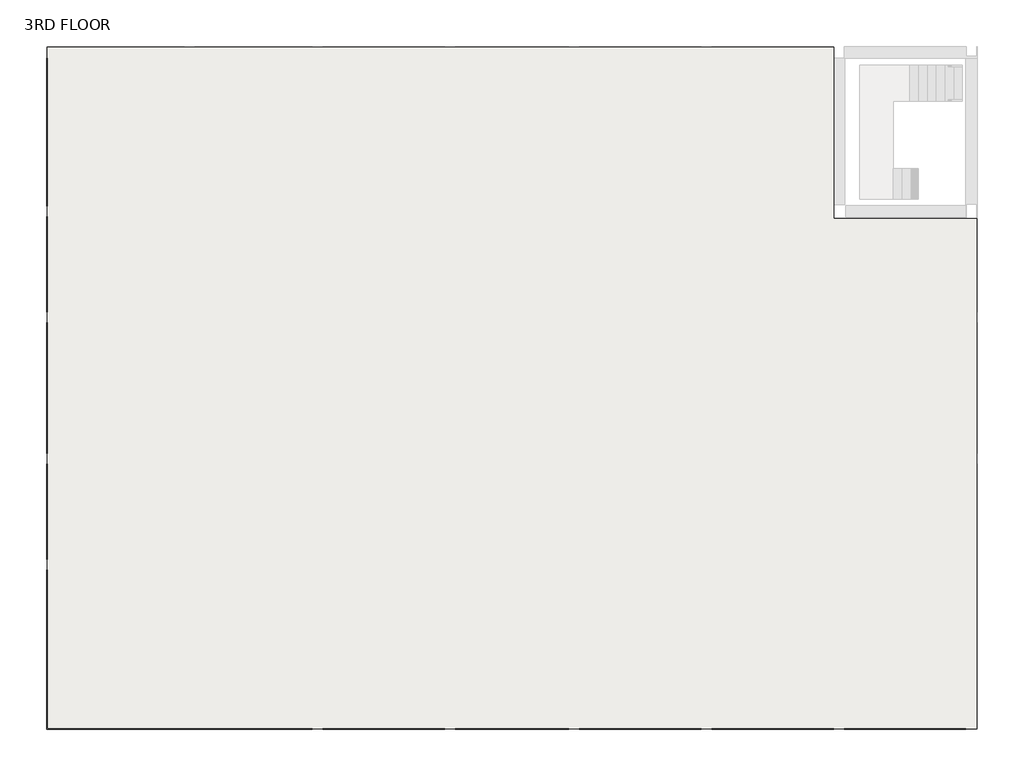
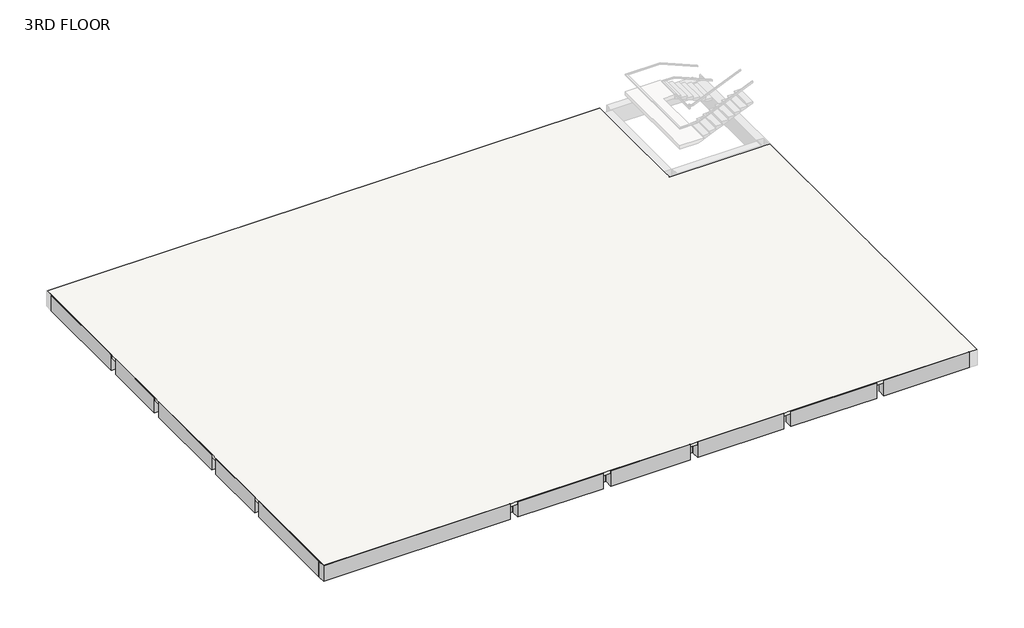
# One storey, part 1 of 2: 9 beams, 1 slab.
"""IFC4 building model written with IfcOpenShell, lengths in millimetres."""

from ifc_helpers import new_model, si_unit, frame, origin, place, context, project, spatial, polyline, outline, extrude, faceted_brep, element, save

model = new_model("IFC4")

# Units and contexts
model_context = context("Model", 3, world=origin())
ifc_project = project(units=[si_unit("LENGTHUNIT", "METRE", prefix="MILLI")], contexts=[model_context])

# Site, building, storey
site = spatial("IfcSite", under=ifc_project)
building = spatial("IfcBuilding", under=site)
storey = spatial("IfcBuildingStorey", under=building, Name="3RD FLOOR", Elevation=10668.0)

# Beams
placement = place(None, origin())
element("IfcBeam", 1, ObjectType="M_Concrete-Rectangular Beam : 400 x 800mm", at=placement, inside=storey, context=model_context, shape_type="Brep", body=[
    faceted_brep([(-25701.5491019, -6047.8309165, 10668.0), (-25701.5491019, -6447.8309165, 10668.0), (-16535.3491019, -6447.8309165, 10668.0), (-16535.3491019, -6425.6309165, 10668.0), (-25679.3491019, -6425.6309165, 10668.0), (-25679.3491019, -6047.8309165, 10668.0), (-25701.5491019, -6047.8309165, 9868.0), (-25679.3491019, -6047.8309165, 10515.6), (-25301.5491019, -6047.8309165, 10515.6), (-20977.1491019, -6047.8309165, 10515.6), (-20577.1491019, -6047.8309165, 10515.6), (-16557.5491019, -6047.8309165, 10515.6), (-16535.3491019, -6047.8309165, 10515.6), (-16535.3491019, -6047.8309165, 9868.0), (-16557.5491019, -6047.8309165, 9868.0), (-20577.1491019, -6047.8309165, 9868.0), (-20977.1491019, -6047.8309165, 9868.0), (-25301.5491019, -6047.8309165, 9868.0), (-25701.5491019, -6447.8309165, 9868.0), (-16535.3491019, -6447.8309165, 9868.0), (-25323.7491019, -6425.6309165, 9868.0), (-25323.7491019, -6070.0309165, 9868.0), (-25679.3491019, -6070.0309165, 9868.0), (-25679.3491019, -6425.6309165, 9868.0), (-20599.3491019, -6425.6309165, 9868.0), (-20599.3491019, -6070.0309165, 9868.0), (-20954.9491019, -6070.0309165, 9868.0), (-20954.9491019, -6425.6309165, 9868.0), (-25323.7491019, -6425.6309165, 10515.6), (-25323.7491019, -6070.0309165, 10515.6), (-16535.3491019, -6425.6309165, 10515.6), (-20599.3491019, -6425.6309165, 10515.6), (-20954.9491019, -6425.6309165, 10515.6), (-25679.3491019, -6425.6309165, 10515.6), (-25679.3491019, -6070.0309165, 10515.6), (-20599.3491019, -6070.0309165, 10515.6), (-20954.9491019, -6070.0309165, 10515.6)], [[[0, 1, 2, 3, 4, 5]], [[6, 0, 5, 7, 8, 9, 10, 11, 12, 13, 14, 15, 16, 17]], [[18, 6, 17, 16, 15, 14, 13, 19], [20, 21, 22, 23], [24, 25, 26, 27]], [[1, 18, 19, 2]], [[1, 0, 6, 18]], [[21, 20, 28, 29]], [[30, 31, 24, 27, 32, 28, 20, 23, 33, 4, 3]], [[4, 33, 23, 22, 34, 7, 5]], [[22, 21, 29, 34]], [[25, 24, 31, 35]], [[27, 26, 36, 32]], [[26, 25, 35, 36]], [[19, 13, 12, 30, 3, 2]], [[28, 32, 36, 35, 31, 30, 12, 11, 10, 9, 8, 7, 34, 29]]]),
    faceted_brep([(5997.6508981, -6447.8309165, 9868.0), (5997.6508981, -6047.8309165, 9868.0), (5997.6508981, -6047.8309165, 10515.6), (5997.6508981, -6425.6309165, 10515.6), (5997.6508981, -6425.6309165, 10668.0), (5997.6508981, -6447.8309165, 10668.0), (1803.4508981, -6047.8309165, 9868.0), (1803.4508981, -6447.8309165, 9868.0), (1803.4508981, -6447.8309165, 10668.0), (1803.4508981, -6425.6309165, 10668.0), (1803.4508981, -6425.6309165, 10515.6), (1803.4508981, -6047.8309165, 10515.6), (1825.6508981, -6047.8309165, 9868.0), (1825.6508981, -6047.8309165, 10515.6)], [[[0, 1, 2, 3, 4, 5]], [[6, 7, 8, 9, 10, 11]], [[8, 5, 4, 9]], [[1, 12, 6, 11, 13, 2]], [[1, 0, 7, 6, 12]], [[0, 5, 8, 7]], [[10, 3, 2, 13, 11]], [[3, 10, 9, 4]]]),
    faceted_brep([(-16179.7491019, -6047.8309165, 9868.0), (-16179.7491019, -6447.8309165, 9868.0), (-16179.7491019, -6447.8309165, 10668.0), (-16179.7491019, -6425.6309165, 10668.0), (-16179.7491019, -6425.6309165, 10515.6), (-16179.7491019, -6047.8309165, 10515.6), (-11963.3491019, -6447.8309165, 10668.0), (-11963.3491019, -6425.6309165, 10668.0), (-11963.3491019, -6047.8309165, 9868.0), (-11985.5491019, -6047.8309165, 9868.0), (-16157.5491019, -6047.8309165, 9868.0), (-16157.5491019, -6047.8309165, 10515.6), (-11985.5491019, -6047.8309165, 10515.6), (-11963.3491019, -6047.8309165, 10515.6), (-11963.3491019, -6447.8309165, 9868.0), (-11963.3491019, -6425.6309165, 10515.6)], [[[0, 1, 2, 3, 4, 5]], [[2, 6, 7, 3]], [[8, 9, 10, 0, 5, 11, 12, 13]], [[1, 0, 10, 9, 8, 14]], [[2, 1, 14, 6]], [[14, 8, 13, 15, 7, 6]], [[15, 4, 3, 7]], [[4, 15, 13, 12, 11, 5]]]),
    faceted_brep([(-11607.7491019, -6047.8309165, 9868.0), (-11607.7491019, -6447.8309165, 9868.0), (-11607.7491019, -6447.8309165, 10668.0), (-11607.7491019, -6425.6309165, 10668.0), (-11607.7491019, -6425.6309165, 10515.6), (-11607.7491019, -6047.8309165, 10515.6), (-7696.1491019, -6447.8309165, 10668.0), (-7696.1491019, -6425.6309165, 10668.0), (-7696.1491019, -6047.8309165, 9868.0), (-7718.3491019, -6047.8309165, 9868.0), (-11585.5491019, -6047.8309165, 9868.0), (-11585.5491019, -6047.8309165, 10515.6), (-7718.3491019, -6047.8309165, 10515.6), (-7696.1491019, -6047.8309165, 10515.6), (-7696.1491019, -6447.8309165, 9868.0), (-7696.1491019, -6425.6309165, 10515.6)], [[[0, 1, 2, 3, 4, 5]], [[2, 6, 7, 3]], [[8, 9, 10, 0, 5, 11, 12, 13]], [[1, 0, 10, 9, 8, 14]], [[2, 1, 14, 6]], [[14, 8, 13, 15, 7, 6]], [[15, 4, 3, 7]], [[4, 15, 13, 12, 11, 5]]]),
    faceted_brep([(-7340.5491019, -6047.8309165, 9868.0), (-7340.5491019, -6447.8309165, 9868.0), (-7340.5491019, -6447.8309165, 10668.0), (-7340.5491019, -6425.6309165, 10668.0), (-7340.5491019, -6425.6309165, 10515.6), (-7340.5491019, -6047.8309165, 10515.6), (-3124.1491019, -6447.8309165, 10668.0), (-3124.1491019, -6425.6309165, 10668.0), (-3124.1491019, -6047.8309165, 9868.0), (-3146.3491019, -6047.8309165, 9868.0), (-7318.3491019, -6047.8309165, 9868.0), (-7318.3491019, -6047.8309165, 10515.6), (-3146.3491019, -6047.8309165, 10515.6), (-3124.1491019, -6047.8309165, 10515.6), (-3124.1491019, -6447.8309165, 9868.0), (-3124.1491019, -6425.6309165, 10515.6)], [[[0, 1, 2, 3, 4, 5]], [[2, 6, 7, 3]], [[8, 9, 10, 0, 5, 11, 12, 13]], [[1, 0, 10, 9, 8, 14]], [[2, 1, 14, 6]], [[14, 8, 13, 15, 7, 6]], [[15, 4, 3, 7]], [[4, 15, 13, 12, 11, 5]]]),
    faceted_brep([(-2768.5491019, -6047.8309165, 9868.0), (-2768.5491019, -6447.8309165, 9868.0), (-2768.5491019, -6447.8309165, 10668.0), (-2768.5491019, -6425.6309165, 10668.0), (-2768.5491019, -6425.6309165, 10515.6), (-2768.5491019, -6047.8309165, 10515.6), (1447.8508981, -6447.8309165, 10668.0), (1447.8508981, -6425.6309165, 10668.0), (1447.8508981, -6047.8309165, 9868.0), (1425.6508981, -6047.8309165, 9868.0), (-2746.3491019, -6047.8309165, 9868.0), (-2746.3491019, -6047.8309165, 10515.6), (1425.6508981, -6047.8309165, 10515.6), (1447.8508981, -6047.8309165, 10515.6), (1447.8508981, -6447.8309165, 9868.0), (1447.8508981, -6425.6309165, 10515.6)], [[[0, 1, 2, 3, 4, 5]], [[2, 6, 7, 3]], [[8, 9, 10, 0, 5, 11, 12, 13]], [[1, 0, 10, 9, 8, 14]], [[2, 1, 14, 6]], [[14, 8, 13, 15, 7, 6]], [[15, 4, 3, 7]], [[4, 15, 13, 12, 11, 5]]]),
])
element("IfcBeam", 2, ObjectType="M_Concrete-Rectangular Beam : 400 x 800mm", at=placement, inside=storey, context=model_context, shape_type="Brep", body=[
    faceted_brep([(-25701.5491019, -939.2309165, 10668.0), (-25701.5491019, -6047.8309165, 10668.0), (-25679.3491019, -6047.8309165, 10668.0), (-25679.3491019, -939.2309165, 10668.0), (-25301.5491019, -6047.8309165, 9868.0), (-25301.5491019, -961.4309165, 9868.0), (-25301.5491019, -939.2309165, 9868.0), (-25301.5491019, -939.2309165, 10515.6), (-25301.5491019, -961.4309165, 10515.6), (-25301.5491019, -6047.8309165, 10515.6), (-25701.5491019, -6047.8309165, 9868.0), (-25701.5491019, -939.2309165, 9868.0), (-25679.3491019, -6047.8309165, 10515.6), (-25679.3491019, -939.2309165, 10515.6)], [[[0, 1, 2, 3]], [[4, 5, 6, 7, 8, 9]], [[4, 10, 11, 6, 5]], [[10, 1, 0, 11]], [[10, 4, 9, 12, 2, 1]], [[6, 11, 0, 3, 13, 7]], [[12, 13, 3, 2]], [[13, 12, 9, 8, 7]]]),
    faceted_brep([(-25301.5491019, 16716.9690835, 9868.0), (-25701.5491019, 16716.9690835, 9868.0), (-25701.5491019, 16716.9690835, 10668.0), (-25679.3491019, 16716.9690835, 10668.0), (-25679.3491019, 16716.9690835, 10515.6), (-25301.5491019, 16716.9690835, 10515.6), (-25701.5491019, 11608.3690835, 10668.0), (-25679.3491019, 11608.3690835, 10668.0), (-25301.5491019, 11608.3690835, 9868.0), (-25301.5491019, 11630.5690835, 9868.0), (-25301.5491019, 11630.5690835, 10515.6), (-25301.5491019, 11608.3690835, 10515.6), (-25701.5491019, 11608.3690835, 9868.0), (-25679.3491019, 11608.3690835, 10515.6)], [[[0, 1, 2, 3, 4, 5]], [[2, 6, 7, 3]], [[8, 9, 0, 5, 10, 11]], [[1, 0, 9, 8, 12]], [[2, 1, 12, 6]], [[12, 8, 11, 13, 7, 6]], [[4, 13, 11, 10, 5]], [[13, 4, 3, 7]]]),
    faceted_brep([(-25701.5491019, 7950.7690835, 9868.0), (-25301.5491019, 7950.7690835, 9868.0), (-25301.5491019, 7950.7690835, 10515.6), (-25679.3491019, 7950.7690835, 10515.6), (-25679.3491019, 7950.7690835, 10668.0), (-25701.5491019, 7950.7690835, 10668.0), (-25301.5491019, 11252.7690835, 9868.0), (-25701.5491019, 11252.7690835, 9868.0), (-25701.5491019, 11252.7690835, 10668.0), (-25679.3491019, 11252.7690835, 10668.0), (-25679.3491019, 11252.7690835, 10515.6), (-25301.5491019, 11252.7690835, 10515.6), (-25301.5491019, 7972.9690835, 10515.6), (-25301.5491019, 11230.5690835, 10515.6), (-25301.5491019, 7972.9690835, 9868.0), (-25301.5491019, 11230.5690835, 9868.0)], [[[0, 1, 2, 3, 4, 5]], [[6, 7, 8, 9, 10, 11]], [[10, 3, 2, 12, 13, 11]], [[3, 10, 9, 4]], [[8, 5, 4, 9]], [[1, 14, 15, 6, 11, 13, 12, 2]], [[1, 0, 7, 6, 15, 14]], [[0, 5, 8, 7]]]),
    faceted_brep([(-25301.5491019, 7595.1690835, 9868.0), (-25701.5491019, 7595.1690835, 9868.0), (-25701.5491019, 7595.1690835, 10668.0), (-25679.3491019, 7595.1690835, 10668.0), (-25679.3491019, 7595.1690835, 10515.6), (-25301.5491019, 7595.1690835, 10515.6), (-25701.5491019, 3073.9690835, 9868.0), (-25301.5491019, 3073.9690835, 9868.0), (-25301.5491019, 3073.9690835, 10515.6), (-25679.3491019, 3073.9690835, 10515.6), (-25679.3491019, 3073.9690835, 10668.0), (-25701.5491019, 3073.9690835, 10668.0), (-25301.5491019, 3096.1690835, 10515.6), (-25301.5491019, 7572.9690835, 10515.6), (-25301.5491019, 3096.1690835, 9868.0), (-25301.5491019, 7572.9690835, 9868.0)], [[[0, 1, 2, 3, 4, 5]], [[6, 7, 8, 9, 10, 11]], [[4, 9, 8, 12, 13, 5]], [[9, 4, 3, 10]], [[2, 11, 10, 3]], [[7, 14, 15, 0, 5, 13, 12, 8]], [[1, 0, 15, 14, 7, 6]], [[2, 1, 6, 11]]]),
    faceted_brep([(-25301.5491019, 2718.3690835, 9868.0), (-25701.5491019, 2718.3690835, 9868.0), (-25701.5491019, 2718.3690835, 10668.0), (-25679.3491019, 2718.3690835, 10668.0), (-25679.3491019, 2718.3690835, 10515.6), (-25301.5491019, 2718.3690835, 10515.6), (-25701.5491019, -583.6309165, 9868.0), (-25301.5491019, -583.6309165, 9868.0), (-25301.5491019, -583.6309165, 10515.6), (-25679.3491019, -583.6309165, 10515.6), (-25679.3491019, -583.6309165, 10668.0), (-25701.5491019, -583.6309165, 10668.0), (-25301.5491019, -561.4309165, 10515.6), (-25301.5491019, 2696.1690835, 10515.6), (-25301.5491019, -561.4309165, 9868.0), (-25301.5491019, 2696.1690835, 9868.0)], [[[0, 1, 2, 3, 4, 5]], [[6, 7, 8, 9, 10, 11]], [[4, 9, 8, 12, 13, 5]], [[9, 4, 3, 10]], [[2, 11, 10, 3]], [[7, 14, 15, 0, 5, 13, 12, 8]], [[0, 15, 14, 7, 6, 1]], [[11, 2, 1, 6]]]),
])
element("IfcBeam", 3, ObjectType="M_Concrete-Rectangular Beam : 400 x 800mm", at=placement, inside=storey, context=model_context, shape_type="SweptSolid", body=[
    extrude(outline(polyline([(-20577.1491019, -6047.8309165), (-20977.1491019, -6047.8309165), (-20977.1491019, -990.0309165), (-20577.1491019, -990.0309165), (-20577.1491019, -6047.8309165)])), frame((0.0, 0.0, 9868.0), z_axis=(0.0, 0.0, 1.0), x_axis=(1.0, 0.0, 0.0)), (0.0, 0.0, 1.0), 647.6),
    extrude(outline(polyline([(-20599.3491019, 16716.9690835), (-20577.1491019, 16716.9690835), (-20577.1491019, 11659.1690835), (-20977.1491019, 11659.1690835), (-20977.1491019, 16716.9690835), (-20954.9491019, 16716.9690835), (-20954.9491019, 16662.9690835), (-20599.3491019, 16662.9690835), (-20599.3491019, 16716.9690835)])), frame((0.0, 0.0, 9868.0), z_axis=(0.0, 0.0, 1.0), x_axis=(1.0, 0.0, 0.0)), (0.0, 0.0, 1.0), 647.6),
    extrude(outline(polyline([(-20977.1491019, 11201.9690835), (-20577.1491019, 11201.9690835), (-20577.1491019, 8001.5690835), (-20977.1491019, 8001.5690835), (-20977.1491019, 11201.9690835)])), frame((0.0, 0.0, 9868.0), z_axis=(0.0, 0.0, 1.0), x_axis=(1.0, 0.0, 0.0)), (0.0, 0.0, 1.0), 647.6),
    extrude(outline(polyline([(-20977.1491019, 7544.3690835), (-20577.1491019, 7544.3690835), (-20577.1491019, 3124.7690835), (-20977.1491019, 3124.7690835), (-20977.1491019, 7544.3690835)])), frame((0.0, 0.0, 9868.0), z_axis=(0.0, 0.0, 1.0), x_axis=(1.0, 0.0, 0.0)), (0.0, 0.0, 1.0), 647.6),
    extrude(outline(polyline([(-20977.1491019, 2667.5690835), (-20577.1491019, 2667.5690835), (-20577.1491019, -532.8309165), (-20977.1491019, -532.8309165), (-20977.1491019, 2667.5690835)])), frame((0.0, 0.0, 9868.0), z_axis=(0.0, 0.0, 1.0), x_axis=(1.0, 0.0, 0.0)), (0.0, 0.0, 1.0), 647.6),
])
element("IfcBeam", 4, ObjectType="M_Concrete-Rectangular Beam : 400 x 800mm", at=placement, inside=storey, context=model_context, shape_type="SweptSolid", body=[
    extrude(outline(polyline([(-16157.5491019, -6047.8309165), (-16179.7491019, -6047.8309165), (-16179.7491019, -6019.2309165), (-16535.3491019, -6019.2309165), (-16535.3491019, -6047.8309165), (-16557.5491019, -6047.8309165), (-16557.5491019, -990.0309165), (-16157.5491019, -990.0309165), (-16157.5491019, -6047.8309165)])), frame((0.0, 0.0, 9868.0), z_axis=(0.0, 0.0, 1.0), x_axis=(1.0, 0.0, 0.0)), (0.0, 0.0, 1.0), 647.6),
    extrude(outline(polyline([(-16179.7491019, 16716.9690835), (-16157.5491019, 16716.9690835), (-16157.5491019, 11659.1690835), (-16557.5491019, 11659.1690835), (-16557.5491019, 16716.9690835), (-16535.3491019, 16716.9690835), (-16535.3491019, 16688.3690835), (-16179.7491019, 16688.3690835), (-16179.7491019, 16716.9690835)])), frame((0.0, 0.0, 9868.0), z_axis=(0.0, 0.0, 1.0), x_axis=(1.0, 0.0, 0.0)), (0.0, 0.0, 1.0), 647.6),
    extrude(outline(polyline([(-16557.5491019, 11201.9690835), (-16157.5491019, 11201.9690835), (-16157.5491019, 8001.5690835), (-16557.5491019, 8001.5690835), (-16557.5491019, 11201.9690835)])), frame((0.0, 0.0, 9868.0), z_axis=(0.0, 0.0, 1.0), x_axis=(1.0, 0.0, 0.0)), (0.0, 0.0, 1.0), 647.6),
    extrude(outline(polyline([(-16557.5491019, 7544.3690835), (-16157.5491019, 7544.3690835), (-16157.5491019, 3124.7690835), (-16557.5491019, 3124.7690835), (-16557.5491019, 7544.3690835)])), frame((0.0, 0.0, 9868.0), z_axis=(0.0, 0.0, 1.0), x_axis=(1.0, 0.0, 0.0)), (0.0, 0.0, 1.0), 647.6),
    extrude(outline(polyline([(-16557.5491019, 2667.5690835), (-16157.5491019, 2667.5690835), (-16157.5491019, -532.8309165), (-16557.5491019, -532.8309165), (-16557.5491019, 2667.5690835)])), frame((0.0, 0.0, 9868.0), z_axis=(0.0, 0.0, 1.0), x_axis=(1.0, 0.0, 0.0)), (0.0, 0.0, 1.0), 647.6),
])
element("IfcBeam", 5, ObjectType="M_Concrete-Rectangular Beam : 400 x 800mm", at=placement, inside=storey, context=model_context, shape_type="SweptSolid", body=[
    extrude(outline(polyline([(-11585.5491019, -6047.8309165), (-11607.7491019, -6047.8309165), (-11607.7491019, -6019.2309165), (-11963.3491019, -6019.2309165), (-11963.3491019, -6047.8309165), (-11985.5491019, -6047.8309165), (-11985.5491019, -990.0309165), (-11585.5491019, -990.0309165), (-11585.5491019, -6047.8309165)])), frame((0.0, 0.0, 9868.0), z_axis=(0.0, 0.0, 1.0), x_axis=(1.0, 0.0, 0.0)), (0.0, 0.0, 1.0), 647.6),
    extrude(outline(polyline([(-11607.7491019, 16716.9690835), (-11585.5491019, 16716.9690835), (-11585.5491019, 11659.1690835), (-11985.5491019, 11659.1690835), (-11985.5491019, 16716.9690835), (-11963.3491019, 16716.9690835), (-11963.3491019, 16688.3690835), (-11607.7491019, 16688.3690835), (-11607.7491019, 16716.9690835)])), frame((0.0, 0.0, 9868.0), z_axis=(0.0, 0.0, 1.0), x_axis=(1.0, 0.0, 0.0)), (0.0, 0.0, 1.0), 647.6),
    extrude(outline(polyline([(-11985.5491019, 11201.9690835), (-11585.5491019, 11201.9690835), (-11585.5491019, 8001.5690835), (-11985.5491019, 8001.5690835), (-11985.5491019, 11201.9690835)])), frame((0.0, 0.0, 9868.0), z_axis=(0.0, 0.0, 1.0), x_axis=(1.0, 0.0, 0.0)), (0.0, 0.0, 1.0), 647.6),
    extrude(outline(polyline([(-11985.5491019, 7544.3690835), (-11585.5491019, 7544.3690835), (-11585.5491019, 3124.7690835), (-11985.5491019, 3124.7690835), (-11985.5491019, 7544.3690835)])), frame((0.0, 0.0, 9868.0), z_axis=(0.0, 0.0, 1.0), x_axis=(1.0, 0.0, 0.0)), (0.0, 0.0, 1.0), 647.6),
    extrude(outline(polyline([(-11585.5491019, -532.8309165), (-11985.5491019, -532.8309165), (-11985.5491019, 2667.5690835), (-11585.5491019, 2667.5690835), (-11585.5491019, -532.8309165)])), frame((0.0, 0.0, 9868.0), z_axis=(0.0, 0.0, 1.0), x_axis=(1.0, 0.0, 0.0)), (0.0, 0.0, 1.0), 647.6),
])
element("IfcBeam", 6, ObjectType="M_Concrete-Rectangular Beam : 400 x 800mm", at=placement, inside=storey, context=model_context, shape_type="SweptSolid", body=[
    extrude(outline(polyline([(-7318.3491019, -6047.8309165), (-7340.5491019, -6047.8309165), (-7340.5491019, -6019.2309165), (-7696.1491019, -6019.2309165), (-7696.1491019, -6047.8309165), (-7718.3491019, -6047.8309165), (-7718.3491019, -990.0309165), (-7318.3491019, -990.0309165), (-7318.3491019, -6047.8309165)])), frame((0.0, 0.0, 9868.0), z_axis=(0.0, 0.0, 1.0), x_axis=(1.0, 0.0, 0.0)), (0.0, 0.0, 1.0), 647.6),
    extrude(outline(polyline([(-7340.5491019, 16716.9690835), (-7318.3491019, 16716.9690835), (-7318.3491019, 11659.1690835), (-7718.3491019, 11659.1690835), (-7718.3491019, 16716.9690835), (-7696.1491019, 16716.9690835), (-7696.1491019, 16688.3690835), (-7340.5491019, 16688.3690835), (-7340.5491019, 16716.9690835)])), frame((0.0, 0.0, 9868.0), z_axis=(0.0, 0.0, 1.0), x_axis=(1.0, 0.0, 0.0)), (0.0, 0.0, 1.0), 647.6),
    extrude(outline(polyline([(-7718.3491019, 7544.3690835), (-7318.3491019, 7544.3690835), (-7318.3491019, 3124.7690835), (-7718.3491019, 3124.7690835), (-7718.3491019, 7544.3690835)])), frame((0.0, 0.0, 9868.0), z_axis=(0.0, 0.0, 1.0), x_axis=(1.0, 0.0, 0.0)), (0.0, 0.0, 1.0), 647.6),
    extrude(outline(polyline([(-7318.3491019, 8001.5690835), (-7718.3491019, 8001.5690835), (-7718.3491019, 11201.9690835), (-7318.3491019, 11201.9690835), (-7318.3491019, 8001.5690835)])), frame((0.0, 0.0, 9868.0), z_axis=(0.0, 0.0, 1.0), x_axis=(1.0, 0.0, 0.0)), (0.0, 0.0, 1.0), 647.6),
    extrude(outline(polyline([(-7318.3491019, -532.8309165), (-7718.3491019, -532.8309165), (-7718.3491019, 2667.5690835), (-7318.3491019, 2667.5690835), (-7318.3491019, -532.8309165)])), frame((0.0, 0.0, 9868.0), z_axis=(0.0, 0.0, 1.0), x_axis=(1.0, 0.0, 0.0)), (0.0, 0.0, 1.0), 647.6),
])
element("IfcBeam", 7, ObjectType="M_Concrete-Rectangular Beam : 400 x 800mm", at=placement, inside=storey, context=model_context, shape_type="SweptSolid", body=[
    extrude(outline(polyline([(-25301.5491019, 3073.9690835), (-25301.5491019, 3096.1690835), (-21005.7491019, 3096.1690835), (-21005.7491019, 2696.1690835), (-25301.5491019, 2696.1690835), (-25301.5491019, 2718.3690835), (-25272.9491019, 2718.3690835), (-25272.9491019, 3073.9690835), (-25301.5491019, 3073.9690835)])), frame((0.0, 0.0, 9868.0), z_axis=(0.0, 0.0, 1.0), x_axis=(1.0, 0.0, 0.0)), (0.0, 0.0, 1.0), 647.6),
    extrude(outline(polyline([(5997.6508981, 3096.1690835), (5997.6508981, 3073.9690835), (5969.0508981, 3073.9690835), (5969.0508981, 2718.3690835), (5997.6508981, 2718.3690835), (5997.6508981, 2696.1690835), (1854.2508981, 2696.1690835), (1854.2508981, 3096.1690835), (5997.6508981, 3096.1690835)])), frame((0.0, 0.0, 9868.0), z_axis=(0.0, 0.0, 1.0), x_axis=(1.0, 0.0, 0.0)), (0.0, 0.0, 1.0), 647.6),
    extrude(outline(polyline([(-20548.5491019, 2696.1690835), (-20548.5491019, 3096.1690835), (-16586.1491019, 3096.1690835), (-16586.1491019, 2696.1690835), (-20548.5491019, 2696.1690835)])), frame((0.0, 0.0, 9868.0), z_axis=(0.0, 0.0, 1.0), x_axis=(1.0, 0.0, 0.0)), (0.0, 0.0, 1.0), 647.6),
    extrude(outline(polyline([(-16128.9491019, 2696.1690835), (-16128.9491019, 3096.1690835), (-12014.1491019, 3096.1690835), (-12014.1491019, 2696.1690835), (-16128.9491019, 2696.1690835)])), frame((0.0, 0.0, 9868.0), z_axis=(0.0, 0.0, 1.0), x_axis=(1.0, 0.0, 0.0)), (0.0, 0.0, 1.0), 647.6),
    extrude(outline(polyline([(1397.0508981, 3096.1690835), (1397.0508981, 2696.1690835), (-2717.7491019, 2696.1690835), (-2717.7491019, 3096.1690835), (1397.0508981, 3096.1690835)])), frame((0.0, 0.0, 9868.0), z_axis=(0.0, 0.0, 1.0), x_axis=(1.0, 0.0, 0.0)), (0.0, 0.0, 1.0), 647.6),
    extrude(outline(polyline([(-3174.9491019, 3096.1690835), (-3174.9491019, 2696.1690835), (-7289.7491019, 2696.1690835), (-7289.7491019, 3096.1690835), (-3174.9491019, 3096.1690835)])), frame((0.0, 0.0, 9868.0), z_axis=(0.0, 0.0, 1.0), x_axis=(1.0, 0.0, 0.0)), (0.0, 0.0, 1.0), 647.6),
    extrude(outline(polyline([(-7746.9491019, 3096.1690835), (-7746.9491019, 2696.1690835), (-11556.9491019, 2696.1690835), (-11556.9491019, 3096.1690835), (-7746.9491019, 3096.1690835)])), frame((0.0, 0.0, 9868.0), z_axis=(0.0, 0.0, 1.0), x_axis=(1.0, 0.0, 0.0)), (0.0, 0.0, 1.0), 647.6),
])
element("IfcBeam", 8, ObjectType="M_Concrete-Rectangular Beam : 400 x 800mm", at=placement, inside=storey, context=model_context, shape_type="SweptSolid", body=[
    extrude(outline(polyline([(-25301.5491019, -583.6309165), (-25301.5491019, -561.4309165), (-21005.7491019, -561.4309165), (-21005.7491019, -961.4309165), (-25301.5491019, -961.4309165), (-25301.5491019, -939.2309165), (-25247.5491019, -939.2309165), (-25247.5491019, -583.6309165), (-25301.5491019, -583.6309165)])), frame((0.0, 0.0, 9868.0), z_axis=(0.0, 0.0, 1.0), x_axis=(1.0, 0.0, 0.0)), (0.0, 0.0, 1.0), 647.6),
    extrude(outline(polyline([(5997.6508981, -561.4309165), (5997.6508981, -961.4309165), (1854.2508981, -961.4309165), (1854.2508981, -561.4309165), (5997.6508981, -561.4309165)])), frame((0.0, 0.0, 9868.0), z_axis=(0.0, 0.0, 1.0), x_axis=(1.0, 0.0, 0.0)), (0.0, 0.0, 1.0), 647.6),
    extrude(outline(polyline([(-20548.5491019, -961.4309165), (-20548.5491019, -561.4309165), (-16586.1491019, -561.4309165), (-16586.1491019, -961.4309165), (-20548.5491019, -961.4309165)])), frame((0.0, 0.0, 9868.0), z_axis=(0.0, 0.0, 1.0), x_axis=(1.0, 0.0, 0.0)), (0.0, 0.0, 1.0), 647.6),
    extrude(outline(polyline([(-16128.9491019, -961.4309165), (-16128.9491019, -561.4309165), (-12014.1491019, -561.4309165), (-12014.1491019, -961.4309165), (-16128.9491019, -961.4309165)])), frame((0.0, 0.0, 9868.0), z_axis=(0.0, 0.0, 1.0), x_axis=(1.0, 0.0, 0.0)), (0.0, 0.0, 1.0), 647.6),
    extrude(outline(polyline([(-11556.9491019, -961.4309165), (-11556.9491019, -561.4309165), (-7746.9491019, -561.4309165), (-7746.9491019, -961.4309165), (-11556.9491019, -961.4309165)])), frame((0.0, 0.0, 9868.0), z_axis=(0.0, 0.0, 1.0), x_axis=(1.0, 0.0, 0.0)), (0.0, 0.0, 1.0), 647.6),
    extrude(outline(polyline([(-7289.7491019, -961.4309165), (-7289.7491019, -561.4309165), (-3174.9491019, -561.4309165), (-3174.9491019, -961.4309165), (-7289.7491019, -961.4309165)])), frame((0.0, 0.0, 9868.0), z_axis=(0.0, 0.0, 1.0), x_axis=(1.0, 0.0, 0.0)), (0.0, 0.0, 1.0), 647.6),
    extrude(outline(polyline([(-2717.7491019, -961.4309165), (-2717.7491019, -561.4309165), (1397.0508981, -561.4309165), (1397.0508981, -961.4309165), (-2717.7491019, -961.4309165)])), frame((0.0, 0.0, 9868.0), z_axis=(0.0, 0.0, 1.0), x_axis=(1.0, 0.0, 0.0)), (0.0, 0.0, 1.0), 647.6),
])
element("IfcBeam", 9, ObjectType="M_Concrete-Rectangular Beam : 400 x 800mm", at=placement, inside=storey, context=model_context, shape_type="SweptSolid", body=[
    extrude(outline(polyline([(-25301.5491019, 7950.7690835), (-25301.5491019, 7972.9690835), (-21005.7491019, 7972.9690835), (-21005.7491019, 7572.9690835), (-25301.5491019, 7572.9690835), (-25301.5491019, 7595.1690835), (-25272.9491019, 7595.1690835), (-25272.9491019, 7950.7690835), (-25301.5491019, 7950.7690835)])), frame((0.0, 0.0, 9868.0), z_axis=(0.0, 0.0, 1.0), x_axis=(1.0, 0.0, 0.0)), (0.0, 0.0, 1.0), 647.6),
    extrude(outline(polyline([(5997.6508981, 7972.9690835), (5997.6508981, 7950.7690835), (5969.0508981, 7950.7690835), (5969.0508981, 7595.1690835), (5997.6508981, 7595.1690835), (5997.6508981, 7572.9690835), (1854.2508981, 7572.9690835), (1854.2508981, 7972.9690835), (5997.6508981, 7972.9690835)])), frame((0.0, 0.0, 9868.0), z_axis=(0.0, 0.0, 1.0), x_axis=(1.0, 0.0, 0.0)), (0.0, 0.0, 1.0), 647.6),
    extrude(outline(polyline([(-7289.7491019, 7572.9690835), (-7289.7491019, 7972.9690835), (-3174.9491019, 7972.9690835), (-3174.9491019, 7572.9690835), (-7289.7491019, 7572.9690835)])), frame((0.0, 0.0, 9868.0), z_axis=(0.0, 0.0, 1.0), x_axis=(1.0, 0.0, 0.0)), (0.0, 0.0, 1.0), 647.6),
    extrude(outline(polyline([(-7746.9491019, 7972.9690835), (-7746.9491019, 7572.9690835), (-11556.9491019, 7572.9690835), (-11556.9491019, 7972.9690835), (-7746.9491019, 7972.9690835)])), frame((0.0, 0.0, 9868.0), z_axis=(0.0, 0.0, 1.0), x_axis=(1.0, 0.0, 0.0)), (0.0, 0.0, 1.0), 647.6),
    extrude(outline(polyline([(1397.0508981, 7972.9690835), (1397.0508981, 7572.9690835), (-2717.7491019, 7572.9690835), (-2717.7491019, 7972.9690835), (1397.0508981, 7972.9690835)])), frame((0.0, 0.0, 9868.0), z_axis=(0.0, 0.0, 1.0), x_axis=(1.0, 0.0, 0.0)), (0.0, 0.0, 1.0), 647.6),
    extrude(outline(polyline([(-12014.1491019, 7972.9690835), (-12014.1491019, 7572.9690835), (-16128.9491019, 7572.9690835), (-16128.9491019, 7972.9690835), (-12014.1491019, 7972.9690835)])), frame((0.0, 0.0, 9868.0), z_axis=(0.0, 0.0, 1.0), x_axis=(1.0, 0.0, 0.0)), (0.0, 0.0, 1.0), 647.6),
    extrude(outline(polyline([(-16586.1491019, 7972.9690835), (-16586.1491019, 7572.9690835), (-20548.5491019, 7572.9690835), (-20548.5491019, 7972.9690835), (-16586.1491019, 7972.9690835)])), frame((0.0, 0.0, 9868.0), z_axis=(0.0, 0.0, 1.0), x_axis=(1.0, 0.0, 0.0)), (0.0, 0.0, 1.0), 647.6),
])

# Slab
element("IfcSlab", 10, ObjectType="6\" Foundation Slab", at=placement, inside=storey, context=model_context, shape_type="Brep", body=[
    faceted_brep([(6375.4508981, -6425.6309165, 10515.6), (6019.8508981, -6425.6309165, 10515.6), (5997.6508981, -6425.6309165, 10515.6), (1803.4508981, -6425.6309165, 10515.6), (1447.8508981, -6425.6309165, 10515.6), (-2768.5491019, -6425.6309165, 10515.6), (-3124.1491019, -6425.6309165, 10515.6), (-7340.5491019, -6425.6309165, 10515.6), (-7696.1491019, -6425.6309165, 10515.6), (-11607.7491019, -6425.6309165, 10515.6), (-11963.3491019, -6425.6309165, 10515.6), (-16179.7491019, -6425.6309165, 10515.6), (-16535.3491019, -6425.6309165, 10515.6), (-20599.3491019, -6425.6309165, 10515.6), (-20954.9491019, -6425.6309165, 10515.6), (-25323.7491019, -6425.6309165, 10515.6), (-25679.3491019, -6425.6309165, 10515.6), (-25679.3491019, -6070.0309165, 10515.6), (-25679.3491019, -6047.8309165, 10515.6), (-25679.3491019, -939.2309165, 10515.6), (-25679.3491019, -583.6309165, 10515.6), (-25679.3491019, 2718.3690835, 10515.6), (-25679.3491019, 3073.9690835, 10515.6), (-25679.3491019, 7595.1690835, 10515.6), (-25679.3491019, 7950.7690835, 10515.6), (-25679.3491019, 11252.7690835, 10515.6), (-25679.3491019, 11608.3690835, 10515.6), (-25679.3491019, 16716.9690835, 10515.6), (-25679.3491019, 16739.1690835, 10515.6), (-25679.3491019, 17094.7690835, 10515.6), (-25323.7491019, 17094.7690835, 10515.6), (-20954.9491019, 17094.7690835, 10515.6), (-20599.3491019, 17094.7690835, 10515.6), (-16535.3491019, 17094.7690835, 10515.6), (-16179.7491019, 17094.7690835, 10515.6), (-11963.3491019, 17094.7690835, 10515.6), (-11607.7491019, 17094.7690835, 10515.6), (-7696.1491019, 17094.7690835, 10515.6), (-7340.5491019, 17094.7690835, 10515.6), (-3124.1491019, 17094.7690835, 10515.6), (-2768.5491019, 17094.7690835, 10515.6), (1447.8508981, 17094.7690835, 10515.6), (1447.8508981, 16716.9690835, 10515.6), (1447.8508981, 16713.7690835, 10515.6), (1447.8508981, 11659.1690835, 10515.6), (1447.8508981, 11201.9690835, 10515.6), (1447.8508981, 11176.5690835, 10515.6), (1825.6508981, 11176.5690835, 10515.6), (5997.6508981, 11176.5690835, 10515.6), (6019.8508981, 11176.5690835, 10515.6), (6375.4508981, 11176.5690835, 10515.6), (6375.4508981, 7950.7690835, 10515.6), (6375.4508981, 7595.1690835, 10515.6), (6375.4508981, 3073.9690835, 10515.6), (6375.4508981, 2718.3690835, 10515.6), (6375.4508981, -507.4309165, 10515.6), (6375.4508981, -1015.4309165, 10515.6), (6375.4508981, -6070.0309165, 10515.6), (-25679.3491019, -6425.6309165, 10668.0), (-16535.3491019, -6425.6309165, 10668.0), (-16179.7491019, -6425.6309165, 10668.0), (-11963.3491019, -6425.6309165, 10668.0), (-11607.7491019, -6425.6309165, 10668.0), (-7696.1491019, -6425.6309165, 10668.0), (-7340.5491019, -6425.6309165, 10668.0), (-3124.1491019, -6425.6309165, 10668.0), (-2768.5491019, -6425.6309165, 10668.0), (1447.8508981, -6425.6309165, 10668.0), (1803.4508981, -6425.6309165, 10668.0), (5997.6508981, -6425.6309165, 10668.0), (6375.4508981, -6425.6309165, 10668.0), (6375.4508981, 2718.3690835, 10668.0), (6375.4508981, 3073.9690835, 10668.0), (6375.4508981, 7595.1690835, 10668.0), (6375.4508981, 7950.7690835, 10668.0), (6375.4508981, 11176.5690835, 10668.0), (6019.8508981, 11176.5690835, 10668.0), (5997.6508981, 11176.5690835, 10668.0), (1825.6508981, 11176.5690835, 10668.0), (1447.8508981, 11176.5690835, 10668.0), (1447.8508981, 11201.9690835, 10668.0), (1447.8508981, 11659.1690835, 10668.0), (1447.8508981, 16713.7690835, 10668.0), (1447.8508981, 17094.7690835, 10668.0), (-2768.5491019, 17094.7690835, 10668.0), (-3124.1491019, 17094.7690835, 10668.0), (-7340.5491019, 17094.7690835, 10668.0), (-7696.1491019, 17094.7690835, 10668.0), (-11607.7491019, 17094.7690835, 10668.0), (-11963.3491019, 17094.7690835, 10668.0), (-16179.7491019, 17094.7690835, 10668.0), (-16535.3491019, 17094.7690835, 10668.0), (-20599.3491019, 17094.7690835, 10668.0), (-20954.9491019, 17094.7690835, 10668.0), (-25679.3491019, 17094.7690835, 10668.0), (-25679.3491019, 16716.9690835, 10668.0), (-25679.3491019, 11608.3690835, 10668.0), (-25679.3491019, 11252.7690835, 10668.0), (-25679.3491019, 7950.7690835, 10668.0), (-25679.3491019, 7595.1690835, 10668.0), (-25679.3491019, 3073.9690835, 10668.0), (-25679.3491019, 2718.3690835, 10668.0), (-25679.3491019, -583.6309165, 10668.0), (-25679.3491019, -939.2309165, 10668.0), (-25679.3491019, -6047.8309165, 10668.0)], [[[0, 1, 2, 3, 4, 5, 6, 7, 8, 9, 10, 11, 12, 13, 14, 15, 16, 17, 18, 19, 20, 21, 22, 23, 24, 25, 26, 27, 28, 29, 30, 31, 32, 33, 34, 35, 36, 37, 38, 39, 40, 41, 42, 43, 44, 45, 46, 47, 48, 49, 50, 51, 52, 53, 54, 55, 56, 57]], [[58, 59, 60, 61, 62, 63, 64, 65, 66, 67, 68, 69, 70, 71, 72, 73, 74, 75, 76, 77, 78, 79, 80, 81, 82, 83, 84, 85, 86, 87, 88, 89, 90, 91, 92, 93, 94, 95, 96, 97, 98, 99, 100, 101, 102, 103, 104]], [[70, 0, 57, 56, 55, 54, 53, 52, 51, 50, 75, 74, 73, 72, 71]], [[16, 15, 14, 13, 12, 11, 10, 9, 8, 7, 6, 5, 4, 3, 2, 1, 0, 70, 69, 68, 67, 66, 65, 64, 63, 62, 61, 60, 59, 58]], [[29, 28, 27, 26, 25, 24, 23, 22, 21, 20, 19, 18, 17, 16, 58, 104, 103, 102, 101, 100, 99, 98, 97, 96, 95, 94]], [[29, 94, 93, 92, 91, 90, 89, 88, 87, 86, 85, 84, 83, 41, 40, 39, 38, 37, 36, 35, 34, 33, 32, 31, 30]], [[79, 46, 45, 44, 43, 42, 41, 83, 82, 81, 80]], [[46, 79, 78, 77, 76, 75, 50, 49, 48, 47]]]),
])

save(model, "model.ifc")

# Revit data of these elements
# Type "M_Concrete-Rectangular Beam : 400 x 800mm"
#   Length [instance default] = 5' - 0"
#   b = 1' - 3.74803"
#   h = 2' - 7.49606"
#   Structural Material [instance default] = Concrete, Cast-in-Place gray
#   Assembly Code = ""
# Type "6\" Foundation Slab"
#   Layers, outside or top first: 0' - 6" "Concrete, Cast-in-Place gray" (function 1)
# Elements 1, 2 (IfcBeam, "M_Concrete-Rectangular Beam : 400 x 800mm")
#   Structural Material = Concrete, Cast-in-Place gray
#   Phase Created = New Construction
#   Materials on its faces: "Concrete, Cast-in-Place gray"
# Elements 3, 4, 5, 6, 7, 8, 9 (IfcBeam, "M_Concrete-Rectangular Beam : 400 x 800mm")
#   Comments = ""
#   Structural Material = Concrete, Cast-in-Place gray
#   Phase Created = New Construction
#   Materials on its faces: "Concrete, Cast-in-Place gray"
# Element 10 (IfcSlab, "6\" Foundation Slab")
#   Height Offset From Level = 0' - 0"
#   built-in parameter 1001954 = 1
#   Phase Created = New Construction
#   Materials on its faces: "Concrete, Cast-in-Place gray"
# Materials
#   "Concrete, Cast-in-Place gray": class "Concrete", colour RGB 192 192 192, transparency 0, Description = "Cast-in-place concrete", Cost = 0
